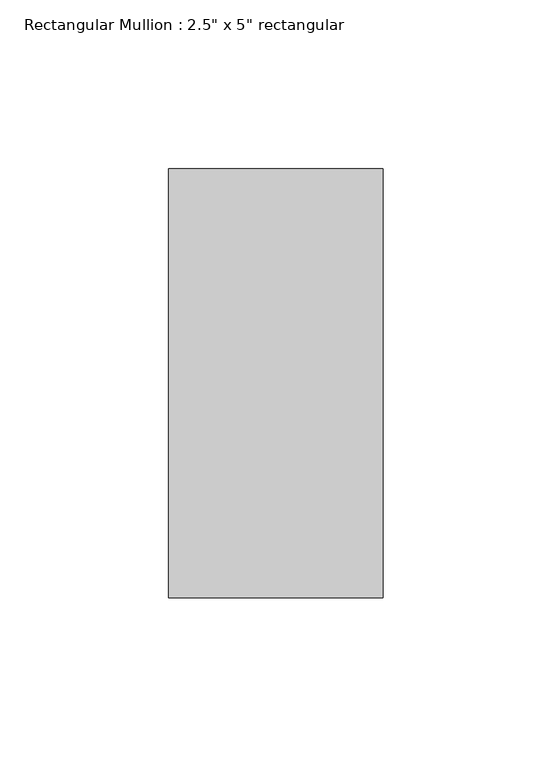
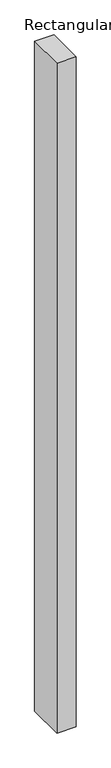
"""IFC4 building model written with IfcOpenShell, lengths in millimetres: member geometry."""

from ifc_helpers import new_model, si_unit, frame, origin, place, context, project, spatial, polyline, outline, extrude, source, transform, mapped, element, save


def member_239fd6c5(model_context):
    return source(origin(), model_context, "Body", "SweptSolid", [
        extrude(outline(polyline([(31.75, 63.5), (31.75, -63.5), (-31.75, -63.5), (-31.75, 63.5), (31.75, 63.5)])), frame((0.0, 0.0, -2343.9308081), z_axis=(0.0, 0.0, 1.0), x_axis=(1.0, 0.0, 0.0)), (0.0, 0.0, 1.0), 2343.9308081),
    ])


if __name__ == "__main__":
    model = new_model("IFC4")
    model_context = context("Model", 3, world=origin())
    ifc_project = project(units=[si_unit("LENGTHUNIT", "METRE", prefix="MILLI")], contexts=[model_context])
    site = spatial("IfcSite", under=ifc_project)
    building = spatial("IfcBuilding", under=site)
    placement = place(None, origin())
    member_shape = member_239fd6c5(model_context)
    element("IfcMember", 1, ObjectType="Rectangular Mullion : 2.5\" x 5\" rectangular", at=placement, inside=building, context=model_context, shape_type="MappedRepresentation", body=[
        mapped(member_shape, transform((0.0, 0.0, 0.0), x_axis=(1.0, 0.0, 0.0), y_axis=(0.0, 1.0, 0.0), z_axis=(0.0, 0.0, 1.0))),
    ])
    save(model, "model.ifc")

# Revit data of these elements
# Type "Rectangular Mullion : 2.5\" x 5\" rectangular"
#   built-in parameter 1007304 = 0.416667 (stored number, unit not read)
#   built-in parameter 1007301 = 0.104167 (stored number, unit not read)
#   built-in parameter 1007300 = 0.104167 (stored number, unit not read)
# Element 1 (IfcMember, "Rectangular Mullion : 2.5\" x 5\" rectangular")
#   Materials on its faces: "Aluminum"
# Materials
#   "Aluminum": class "Metal", colour RGB 247 247 247, transparency 0, Description = "Aluminum 6061", Cost = 0
